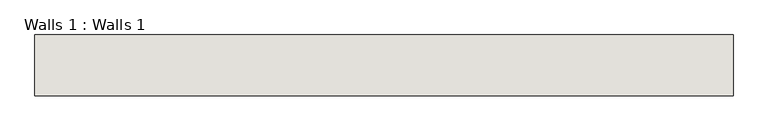
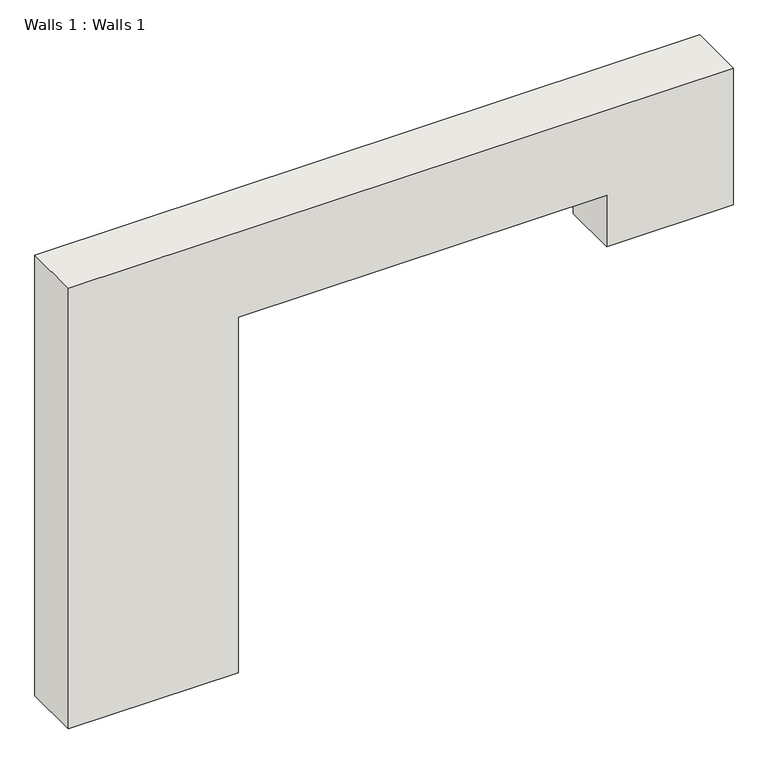
"""IFC4 building model written with IfcOpenShell, lengths in millimetres: wall geometry, Walls 1 : Walls 1."""

from ifc_helpers import new_model, si_unit, frame, origin, place, context, project, spatial, polyline, outline, extrude, source, transform, mapped, element, save


def walls_1_walls_1_0e52aedd(model_context):
    return source(origin(), model_context, "Body", "SweptSolid", [
        extrude(outline(polyline([(-400.0, -17842.4019361), (-400.0, -15456.4019361), (4876.8, -15456.4019361), (4876.8, -10274.8019361), (4114.8, -10274.8019361), (4114.8, -8498.4019361), (6146.8, -8498.4019361), (6146.8, -17842.4019361), (-400.0, -17842.4019361)])), frame((0.0, -7417.452727, 0.0), z_axis=(0.0, 1.0, 0.0), x_axis=(0.0, 0.0, 1.0)), (0.0, 0.0, 1.0), 811.5964357),
    ])


if __name__ == "__main__":
    model = new_model("IFC4")
    model_context = context("Model", 3, world=origin())
    ifc_project = project(units=[si_unit("LENGTHUNIT", "METRE", prefix="MILLI")], contexts=[model_context])
    site = spatial("IfcSite", under=ifc_project)
    building = spatial("IfcBuilding", under=site)
    placement = place(None, origin())
    walls_1_walls_1_shape = walls_1_walls_1_0e52aedd(model_context)
    element("IfcWall", 1, ObjectType="Walls 1 : Walls 1", at=placement, inside=building, context=model_context, shape_type="MappedRepresentation", body=[
        mapped(walls_1_walls_1_shape, transform((0.0, 0.0, 0.0), x_axis=(1.0, 0.0, 0.0), y_axis=(0.0, 1.0, 0.0), z_axis=(0.0, 0.0, 1.0))),
    ])
    save(model, "model.ifc")

# Revit data of these elements
# Element 1 (IfcWall, "Walls 1 : Walls 1")
#   Materials on its faces: "Default Wall"
# Materials
#   "Default Wall": colour RGB 80 80 80, transparency 0
